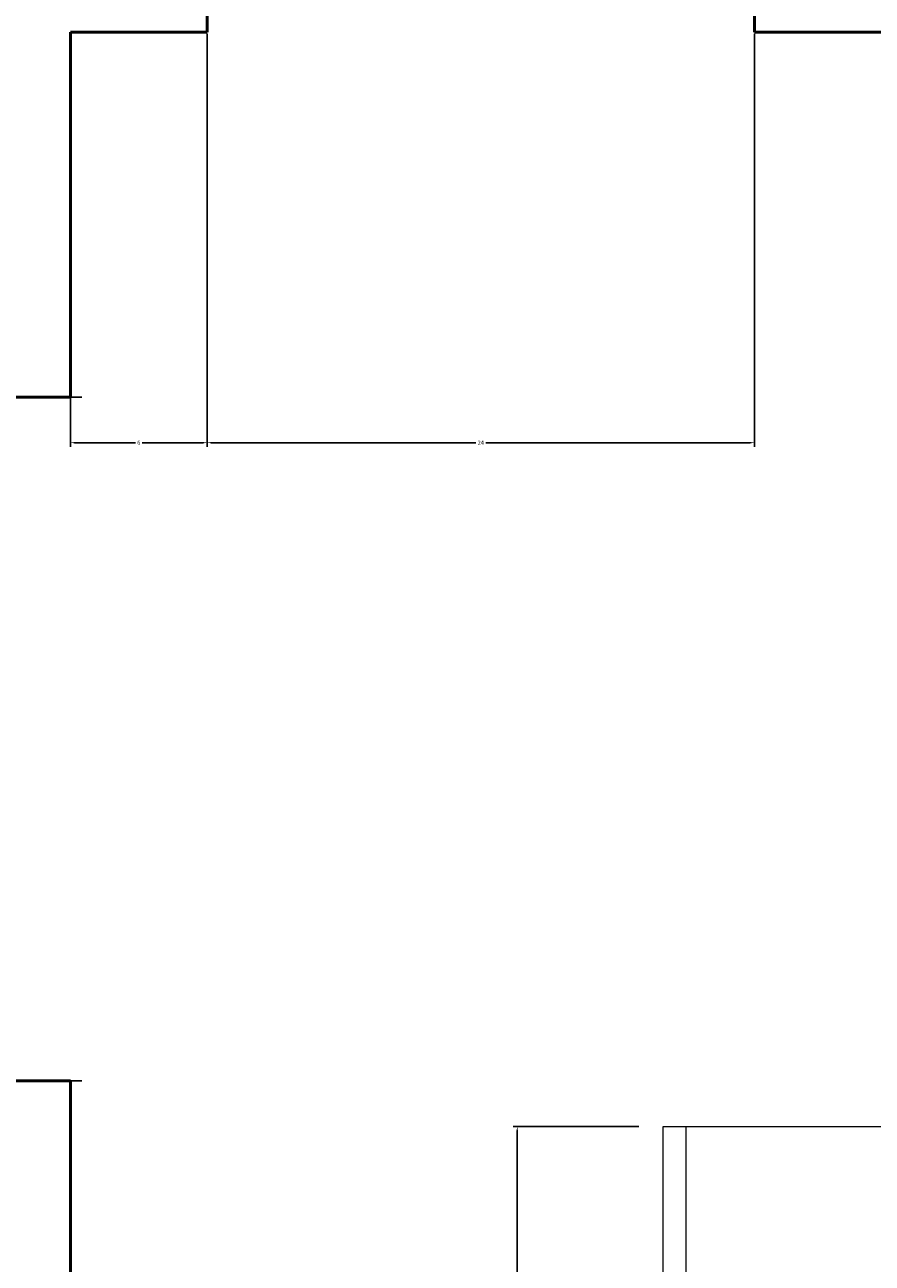
# Model space of a CAD drawing. Units: inches. Extents: x 2621 to 2849, y 2066 to 2463.
# Tile 20 of 28: x 2766 to 2803, y 2317 to 2372. Entities that reach past the tile are written whole.
import ezdxf

# ---------------------------------------------------------------- set-up
doc = ezdxf.new("R2010")
doc.units = ezdxf.units.IN
for name, color, linetype, lineweight in [('A-ANNO-DIMS', 2, 'Continuous', 18), ('A-DOOR', 3, 'Continuous', 25), ('A-EQPM', 8, 'Continuous', 18), ('A-WALL', 7, 'Continuous', 50)]:
    doc.layers.add(name, color=color, linetype=linetype, lineweight=lineweight)
doc.styles.get("Standard").update_dxf_attribs({"font": 'arial.ttf'})
doc.dimstyles.get("Standard").update_dxf_attribs({"dimtxt": 0.18, "dimasz": 0.18, "dimexe": 0.18, "dimexo": 0.0625, "dimgap": 0.09, "dimtad": 0, "dimtih": 1, "dimtoh": 1, "dimdec": 4, "dimzin": 0, "dimdsep": 46, "dimtxsty": 'Standard', "dimcen": 0.09, "dimadec": 0, "dimazin": 0, "dimtfac": 1, "dimtdec": 4, "dimtofl": 0, "dimtmove": 0, "dimatfit": 3, "dimfxl": 1, "dimtolj": 1, "dimtzin": 0, "dimarcsym": 0})

# ---------------------------------------------------------------- blocks, each defined once
blk = doc.blocks.new('Refrigerator-2 door - 36 in top')
for p, q in [((0, -26.999999), (36, -26.999999)), ((12, -26.999999), (12, -28.999999)), ((11, -27.999999), (11, -28.999999)), ((13, -28.999999), (13, -27.999999)), ((11, -28.999999), (13, -28.999999))]:
    blk.add_line(p, q)
blk.add_lwpolyline([(0, -27.999999), (0, 0), (36, 0), (36, -27.999999)], close=True)
blk = doc.blocks.new('*U4')
for p, q in [((0, 0), (0, -6)), ((40, 0), (40, -6))]:
    blk.add_line(p, q)
blk.add_lwpolyline([(0, 0), (34.641, 20), (35.516, 18.484), (0.875, -1.516)], close=True)
blk.add_arc((0, 0), 40, 0, 30)
blk = doc.blocks.new('*U5')
for p, q in [((0, 0), (0, 6)), ((40, 0), (40, 6))]:
    blk.add_line(p, q)
blk.add_lwpolyline([(0, 0), (34.641, -20), (35.516, -18.484), (0.875, 1.516)], close=True)
blk.add_arc((0, 0), 40, 330, 0)
blk = doc.blocks.new('*D17')
at = {"layer": 'A-ANNO-DIMS', "color": 0, "lineweight": -2, "transparency": 16777216}
for p, q in [((2792.808, 2323.375), (2787.29, 2323.375)), ((2787.47, 2323.195), (2787.47, 2305.558)), ((2787.47, 2287.555), (2787.47, 2305.191)), ((2792.808, 2287.375), (2787.29, 2287.375))]:
    blk.add_line(p, q, dxfattribs=at)
at = {"layer": 'A-ANNO-DIMS', "color": 0, "transparency": 16777216}
for points in [[(2787.44, 2323.195), (2787.5, 2323.195), (2787.47, 2323.375)], [(2787.44, 2287.555), (2787.5, 2287.555), (2787.47, 2287.375)]]:
    blk.add_solid(points, dxfattribs=at)
at = {"layer": 'Defpoints', "color": 0, "transparency": 16777216}
for p in [(2792.87, 2323.375), (2787.47, 2287.375), (2792.87, 2287.375)]:
    blk.add_point(p, dxfattribs=at)
at = {"layer": 'A-ANNO-DIMS', "color": 0, "transparency": 16777216, "insert": (2787.47, 2305.375), "char_height": 0.18, "attachment_point": 5}
blk.add_mtext('\\A1;REFRIGERATOR 36', dxfattribs=at)
blk = doc.blocks.new('*D52')
at = {"layer": 'A-ANNO-DIMS', "color": 0, "lineweight": -2, "transparency": 16777216}
for p, q in [((2773.87, 2371.312), (2773.87, 2353.191)), ((2797.87, 2371.312), (2797.87, 2353.191)), ((2774.05, 2353.371), (2785.65, 2353.371)), ((2797.69, 2353.371), (2786.09, 2353.371))]:
    blk.add_line(p, q, dxfattribs=at)
at = {"layer": 'A-ANNO-DIMS', "color": 0, "transparency": 16777216}
for points in [[(2774.05, 2353.401), (2774.05, 2353.341), (2773.87, 2353.371)], [(2797.69, 2353.401), (2797.69, 2353.341), (2797.87, 2353.371)]]:
    blk.add_solid(points, dxfattribs=at)
at = {"layer": 'Defpoints', "color": 0, "transparency": 16777216}
for p in [(2773.87, 2371.375), (2797.87, 2371.375), (2773.87, 2353.371)]:
    blk.add_point(p, dxfattribs=at)
at = {"layer": 'A-ANNO-DIMS', "color": 0, "transparency": 16777216, "insert": (2785.87, 2353.371), "char_height": 0.18, "attachment_point": 5}
blk.add_mtext('\\A1;24', dxfattribs=at)
blk = doc.blocks.new('*D53')
at = {"layer": 'A-ANNO-DIMS', "color": 0, "lineweight": -2, "transparency": 16777216}
for p, q in [((2767.87, 2371.312), (2767.87, 2353.191)), ((2773.87, 2371.312), (2773.87, 2353.191)), ((2768.05, 2353.371), (2770.721, 2353.371)), ((2773.69, 2353.371), (2771.02, 2353.371))]:
    blk.add_line(p, q, dxfattribs=at)
at = {"layer": 'A-ANNO-DIMS', "color": 0, "transparency": 16777216}
for points in [[(2768.05, 2353.401), (2768.05, 2353.341), (2767.87, 2353.371)], [(2773.69, 2353.401), (2773.69, 2353.341), (2773.87, 2353.371)]]:
    blk.add_solid(points, dxfattribs=at)
at = {"layer": 'Defpoints', "color": 0, "transparency": 16777216}
for p in [(2767.87, 2371.375), (2773.87, 2371.375), (2767.87, 2353.371)]:
    blk.add_point(p, dxfattribs=at)
at = {"layer": 'A-ANNO-DIMS', "color": 0, "transparency": 16777216, "insert": (2770.87, 2353.371), "char_height": 0.18, "attachment_point": 5}
blk.add_mtext('\\A1;6', dxfattribs=at)

msp = doc.modelspace()

# ---------------------------------------------------------------- linework, layer by layer
at = {"layer": 'A-WALL'}
for p, q in [((2773.8701, 2375.3746), (2773.8701, 2371.3746)), ((2797.8701, 2375.3746), (2797.8701, 2371.3746)), ((2767.8701, 2371.3746), (2773.8701, 2371.3746)), ((2767.8701, 2355.3746), (2767.8701, 2371.3746)), ((2797.8701, 2371.3746), (2821.8701, 2371.3746)), ((2763.8701, 2355.3746), (2767.8701, 2355.3746)), ((2763.8701, 2325.3746), (2767.8701, 2325.3746)), ((2767.8701, 2315.3746), (2767.8701, 2325.3746))]:
    msp.add_line(p, q, dxfattribs=at)

# ---------------------------------------------------------------- block references
at = {"layer": 'A-DOOR', "xscale": 0.6, "yscale": 0.6, "zscale": 0.6}
msp.add_blockref('*U4', (2773.8701, 2374.9746), dxfattribs=at)
at = {"layer": 'A-DOOR', "xscale": 0.75, "yscale": 0.75, "zscale": 0.75, "rotation": 270}
msp.add_blockref('*U5', (2763.8701, 2355.3746), dxfattribs=at)
at = {"layer": 'A-EQPM', "rotation": 270}
msp.add_blockref('Refrigerator-2 door - 36 in top', (2821.8701, 2323.3746), dxfattribs=at)

# ---------------------------------------------------------------- dimensions: what is measured, and where the dimension line sits
at = {"layer": 'A-ANNO-DIMS'}
for base, p1, p2, picture, middle in [((2767.8701, 2353.3711), (2773.8701, 2371.3746), (2767.8701, 2371.3746), '*D53', (2770.8701, 2353.3711)), ((2773.8701, 2353.3711), (2797.8701, 2371.3746), (2773.8701, 2371.3746), '*D52', (2785.8701, 2353.3711))]:
    dim = msp.add_linear_dim(base=base, p1=p1, p2=p2, angle=180, dimstyle='Standard', override={"dimdec": 0, "dimlfac": 1, "dimrnd": 0, "dimzin": 0, "dimdsep": 46, "dimlunit": 2}, dxfattribs=at)
    dim.commit()
    dim.dimension.update_dxf_attribs({"geometry": picture, "text_midpoint": middle})
dim = msp.add_linear_dim(base=(2787.4701, 2287.3746), p1=(2792.8701, 2323.3746), p2=(2792.8701, 2287.3746), angle=270, text='REFRIGERATOR <>', dimstyle='Standard', override={"dimdec": 0, "dimlfac": 1, "dimrnd": 0, "dimzin": 0, "dimdsep": 46, "dimlunit": 2}, dxfattribs=at)
dim.commit()
dim.dimension.update_dxf_attribs({"geometry": '*D17', "text_midpoint": (2787.4701, 2305.3746)})

doc.saveas('drawing.dxf')
